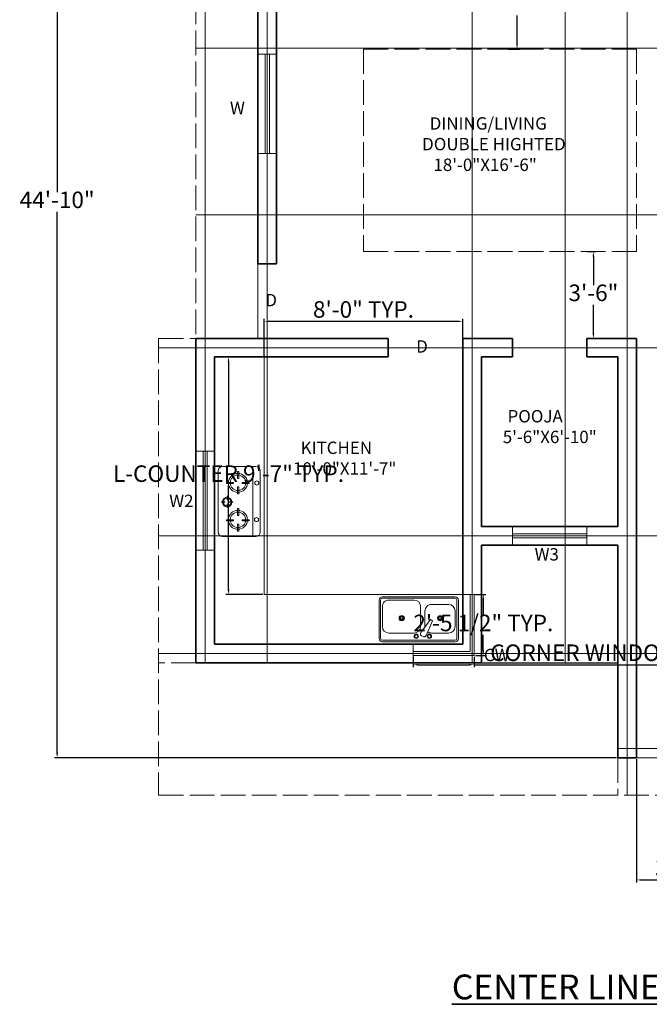
# Model space of a CAD drawing. Units: inches. Extents: x 1070 to 2371, y 645 to 1546.
# Tile 8 of 10: x 1710 to 2015, y 686 to 1162. Entities that reach past the tile are written whole.
import ezdxf

# ---------------------------------------------------------------- set-up
doc = ezdxf.new("R2010")
doc.units = ezdxf.units.IN
doc.linetypes.add('ACAD_ISO02W100', pattern=[15, 12, -3])
for name, color, linetype, lineweight in [('A-ANNO-DIMS', 2, 'Continuous', 18), ('A-ANNO-TEXT', 7, 'Continuous', 18), ('A-ANNO-TITL', 7, 'Continuous', 35), ('A-AREA-IDEN', 7, 'Continuous', 18), ('A-DOOR', 4, 'Continuous', 18), ('A-EQPM', 9, 'Continuous', 18), ('A-FLOR', 7, 'Continuous', 25), ('A-FLOR-CASE', 9, 'Continuous', 18), ('A-FLOR-FIXT', 9, 'Continuous', 18), ('A-FLOR-OVHD', 8, 'ACAD_ISO02W100', 13), ('A-GLAZ', 4, 'Continuous', 18), ('A-GRID', 8, 'Continuous', 13), ('A-ROOF-OVHD', 8, 'ACAD_ISO02W100', 13), ('A-WALL', 7, 'Continuous', 35)]:
    doc.layers.add(name, color=color, linetype=linetype, lineweight=lineweight)
doc.styles.get("Standard").update_dxf_attribs({"font": 'arial.ttf'})
doc.dimstyles.new('ISO-25', dxfattribs={"dimtxt": 8, "dimasz": 2.5, "dimexe": 1.25, "dimexo": 0.625, "dimtad": 1, "dimtih": 1, "dimtoh": 1, "dimdec": 1, "dimlunit": 3, "dimtxsty": 'Standard', "dimcen": 2.5, "dimadec": 0, "dimazin": 0, "dimtfac": 1, "dimtdec": 1, "dimtmove": 0, "dimatfit": 3, "dimfxl": 1, "dimarcsym": 0})

# ---------------------------------------------------------------- blocks, each defined once
blk = doc.blocks.new('A$C51B36FC3')
at = {"linetype": 'ByBlock'}
for p, q in [((0, 421.4), (0, 33)), ((15, 421.4), (15, 33)), ((767.9, 454.4), (33, 454.4)), ((767.9, 439.4), (33, 439.4)), ((357.3, 402.3), (372.7, 393.4)), ((785.9, 33), (785.9, 421.4)), ((800.9, 33), (800.9, 421.4)), ((33, 143.2), (33, 300.3)), ((99.1, 366.3), (271.4, 366.3)), ((325.7, 391), (261.9, 241.3)), ((281, 230.3), (378.7, 360.4)), ((337.5, 299.4), (337.5, 143.2)), ((381.5, 99.1), (381.5, 300.3)), ((447.6, 366.3), (701.8, 366.3)), ((767.9, 300.3), (767.9, 99.1)), ((167.7, 217.2), (157.7, 218.2)), ((167.7, 213.8), (157.8, 212.7)), ((168.5, 220.9), (159, 224.1)), ((168.6, 210), (159.2, 206.6)), ((169.7, 223.8), (161, 228.6)), ((170.1, 206.9), (161.5, 201.7)), ((171.7, 226.6), (164.2, 233.2)), ((172.4, 203.8), (165.3, 196.8)), ((174.6, 229.3), (168.8, 237.4)), ((175, 201.7), (169.3, 193.4)), ((178.2, 231.2), (174.5, 240.5)), ((179.3, 199.6), (176.3, 190.1)), ((181.4, 232.2), (179.7, 242)), ((185.3, 232.4), (185.8, 242.4)), ((188.6, 199.3), (191.1, 189.6)), ((189.3, 231.7), (192.3, 241.3)), ((192, 200.6), (196.5, 191.7)), ((193.1, 230.1), (198.2, 238.7)), ((195.5, 202.9), (202.1, 195.4)), ((196, 227.8), (203, 235)), ((198.3, 206.1), (206.6, 200.5)), ((199, 224.1), (207.6, 229.1)), ((200.1, 209.6), (209.5, 206)), ((200.4, 221), (209.9, 224.1)), ((201, 212.9), (210.9, 211.3)), ((201.2, 216.9), (211.2, 217.6)), ((261.9, 241.3), (281, 230.3)), ((555.9, 217.2), (546, 218.2)), ((556, 213.8), (546, 212.7)), ((556.7, 220.9), (547.2, 224.1)), ((556.8, 210), (547.4, 206.6)), ((558, 223.8), (549.2, 228.6)), ((558.3, 206.9), (549.8, 201.7)), ((560, 226.6), (552.4, 233.2)), ((560.7, 203.8), (553.6, 196.8)), ((562.9, 229.3), (557.1, 237.4)), ((563.2, 201.7), (557.6, 193.4)), ((566.5, 231.2), (562.8, 240.5)), ((567.6, 199.6), (564.5, 190.1)), ((569.7, 232.2), (567.9, 242)), ((573.5, 232.4), (574, 242.4)), ((576.9, 199.3), (579.4, 189.6)), ((577.6, 231.7), (580.5, 241.3)), ((580.3, 200.6), (584.8, 191.7)), ((581.3, 230.1), (586.4, 238.7)), ((583.7, 202.9), (590.3, 195.4)), ((584.3, 227.8), (591.2, 235)), ((586.6, 206.1), (594.8, 200.5)), ((587.2, 224.1), (595.9, 229.1)), ((588.4, 209.6), (597.7, 206)), ((588.6, 221), (598.1, 224.1)), ((589.3, 212.9), (599.2, 211.3)), ((589.5, 216.9), (599.4, 217.6)), ((184.7, 198.8), (184.8, 188.8)), ((572.9, 198.8), (573.1, 188.8)), ((33, 15), (767.9, 15)), ((33, 0), (767.9, 0)), ((271.4, 77.1), (99.1, 77.1)), ((701.8, 33), (447.6, 33))]:
    blk.add_line(p, q, dxfattribs=at)
for centre, radius in [((293.4, 399.4), 22), ((293.4, 399.4), 16), ((425.6, 399.4), 22), ((425.6, 399.4), 16), ((184.4, 215.6), 26.8), ((184.4, 215.6), 16.8), ((184.4, 215.6), 11.8), ((572.7, 215.6), 26.8), ((572.7, 215.6), 16.8), ((572.7, 215.6), 11.8)]:
    blk.add_circle(centre, radius, dxfattribs=at)
for centre, radius, start, end in [((33, 421.4), 33, 90, 180), ((33, 421.4), 18, 90, 180), ((346.3, 383.2), 22, 60, 159.46232), ((767.9, 421.4), 33, 0, 90), ((767.9, 421.4), 18, 0, 90), ((99.1, 300.3), 66.1, 90, 180), ((271.4, 300.3), 66.1, 56.60703, 90), ((361.7, 374.4), 22, 320.53768, 60), ((447.6, 300.3), 66.1, 90, 180), ((701.8, 300.3), 66.1, 0, 90), ((99.1, 143.2), 66.1, 180, 270), ((271.4, 143.2), 66.1, 270, 0), ((33, 33), 33, 180, 270), ((33, 33), 18, 180, 270), ((447.6, 99.1), 66.1, 180, 270), ((701.8, 99.1), 66.1, 270, 0), ((767.9, 33), 33, 270, 0), ((767.9, 33), 18, 270, 0)]:
    blk.add_arc(centre, radius, start, end, dxfattribs=at)
blk = doc.blocks.new('A$C2A3C6842')
for p, q in [((45, 432), (675, 432)), ((0, 45), (0, 387)), ((162, 347), (173, 347)), ((162, 276), (162, 347)), ((173, 347), (173, 276)), ((298, 342), (298, 336)), ((334, 342), (298, 342)), ((298, 336), (334, 336)), ((334, 336), (334, 342)), ((352, 363), (352, 399)), ((352, 399), (357, 399)), ((357, 363), (352, 363)), ((357, 319), (352, 319)), ((352, 319), (352, 283)), ((357, 399), (357, 363)), ((357, 283), (357, 319)), ((379, 336), (379, 342)), ((379, 342), (414, 342)), ((414, 336), (379, 336)), ((414, 342), (414, 336)), ((545, 347), (556, 347)), ((545, 276), (545, 347)), ((556, 347), (556, 276)), ((720, 387), (720, 45)), ((55, 233), (55, 221)), ((127, 233), (55, 233)), ((55, 221), (127, 221)), ((127, 221), (127, 233)), ((173, 276), (162, 276)), ((216, 221), (216, 233)), ((216, 233), (287, 233)), ((287, 221), (216, 221)), ((287, 233), (287, 221)), ((352, 283), (357, 283)), ((438, 233), (438, 221)), ((510, 233), (438, 233)), ((438, 221), (510, 221)), ((510, 221), (510, 233)), ((556, 276), (545, 276)), ((598, 233), (670, 233)), ((598, 221), (598, 233)), ((670, 221), (598, 221)), ((670, 233), (670, 221)), ((173, 187), (162, 187)), ((162, 187), (162, 115)), ((162, 115), (173, 115)), ((173, 115), (173, 187)), ((556, 187), (545, 187)), ((545, 187), (545, 115)), ((545, 115), (556, 115)), ((556, 115), (556, 187)), ((1, 77), (720, 77)), ((675, 0), (45, 0))]:
    blk.add_line(p, q)
at = {"extrusion": (0, -1e-16, -1)}
for centre, major_axis, start_param, end_param in [((45, 387), (31.8, 31.8), 3.926991, 5.497787), ((172, 230), (-97.3, 0.1), -0.001099, 6.282086), ((552, 230), (-97.3, 0.1), -0.001099, 6.282086), ((174, 39), (-14.8, 14.8), 5.497787, 11.780972)]:
    blk.add_ellipse(centre, major_axis=major_axis, ratio=1, start_param=start_param, end_param=end_param, dxfattribs=at)
at = {"extrusion": (0, 1e-16, -1)}
blk.add_ellipse((675, 387), major_axis=(-31.8, 31.8), ratio=1, start_param=0.785398, end_param=2.356194, dxfattribs=at)
at = {"extrusion": (-1e-16, -4e-16, -1)}
for centre in [(172, 230), (552, 230)]:
    blk.add_ellipse(centre, major_axis=(-79.3, 0), ratio=1, start_param=-0.0002116186602152, end_param=6.282973688519371, dxfattribs=at)
at = {"extrusion": (-1e-16, -1e-16, -1)}
blk.add_ellipse((355, 340), major_axis=(48.7, 0.1), ratio=1, start_param=3.144125, end_param=9.42731, dxfattribs=at)
at = {"extrusion": (-1e-16, 0, -1)}
for centre, major_axis, start_param, end_param in [((355, 340), (-39.7, 0), -0.000334, 6.282851), ((45, 45), (-31.8, 31.8), 3.926991, 5.497787)]:
    blk.add_ellipse(centre, major_axis=major_axis, ratio=1, start_param=start_param, end_param=end_param, dxfattribs=at)
at = {"extrusion": (2e-16, -2e-16, -1)}
blk.add_ellipse((551, 36), major_axis=(14.8, 14.8), ratio=1, start_param=3.926991, end_param=10.210176, dxfattribs=at)
at = {"extrusion": (-2e-16, 1e-16, -1)}
blk.add_ellipse((675, 45), major_axis=(31.8, 31.8), ratio=1, start_param=0.785398, end_param=2.356194, dxfattribs=at)
at = {"text_generation_flag": 4, "flags": 9}
for tag in ['XSIZE', 'YSIZE']:
    blk.add_attdef(tag, (361, 265), '', height=0.45, rotation=180, dxfattribs=at)
blk = doc.blocks.new('*D15')
at = {"layer": 'A-ANNO-DIMS', "color": 0, "lineweight": -2, "transparency": 16777216}
for p, q in [((1984.57, 1049.77), (1988.94, 1049.77)), ((1987.69, 1047.27), (1987.69, 1033.48)), ((1987.69, 1010.27), (1987.69, 1024.06)), ((1985.17, 1007.77), (1988.94, 1007.77))]:
    blk.add_line(p, q, dxfattribs=at)
at = {"layer": 'A-ANNO-DIMS', "color": 0, "transparency": 16777216}
for points in [[(1987.28, 1047.27), (1988.11, 1047.27), (1987.69, 1049.77)], [(1987.28, 1010.27), (1988.11, 1010.27), (1987.69, 1007.77)]]:
    blk.add_solid(points, dxfattribs=at)
at = {"layer": 'Defpoints', "color": 0, "transparency": 16777216}
for p in [(1983.94, 1049.77), (1987.69, 1049.77), (1984.54, 1007.77)]:
    blk.add_point(p, dxfattribs=at)
at = {"layer": 'A-ANNO-DIMS', "color": 0, "transparency": 16777216, "insert": (1987.69, 1028.77), "char_height": 8, "attachment_point": 5}
blk.add_mtext('3\'-6"', dxfattribs=at)
blk = doc.blocks.new('*D16')
at = {"layer": 'A-ANNO-DIMS', "color": 0, "lineweight": -2, "transparency": 16777216}
for p, q in [((1946.48, 1189.77), (1952.04, 1189.77)), ((1950.79, 1187.27), (1950.79, 1173.48)), ((1950.79, 1150.27), (1950.79, 1164.06)), ((1946.48, 1147.77), (1952.04, 1147.77))]:
    blk.add_line(p, q, dxfattribs=at)
at = {"layer": 'A-ANNO-DIMS', "color": 0, "transparency": 16777216}
for points in [[(1950.37, 1187.27), (1951.21, 1187.27), (1950.79, 1189.77)], [(1950.37, 1150.27), (1951.21, 1150.27), (1950.79, 1147.77)]]:
    blk.add_solid(points, dxfattribs=at)
at = {"layer": 'Defpoints', "color": 0, "transparency": 16777216}
for p in [(1945.86, 1189.77), (1950.79, 1189.77), (1945.86, 1147.77)]:
    blk.add_point(p, dxfattribs=at)
at = {"layer": 'A-ANNO-DIMS', "color": 0, "transparency": 16777216, "insert": (1950.79, 1168.77), "char_height": 8, "attachment_point": 5}
blk.add_mtext('3\'-6"', dxfattribs=at)
blk = doc.blocks.new('GLAZ-CORNER')
for p, q in [((27.5, 29.5), (27.5, 2)), ((29.5, 29.5), (29.5, 0)), ((0, 2), (27.5, 2)), ((0, 0), (29.5, 0))]:
    blk.add_line(p, q)
blk = doc.blocks.new('GLAZ-36IN')
for p, q in [((0, 2), (36, 2)), ((0, 0), (36, 0))]:
    blk.add_line(p, q)
blk = doc.blocks.new('GLAZ-48IN')
for p, q in [((0, 48), (0, 0)), ((2, 48), (2, 0))]:
    blk.add_line(p, q)
blk = doc.blocks.new('COUNTER-L-KITCHEN')
for p, q in [((0, 115), (0, 0)), ((0, 0), (96, 0))]:
    blk.add_line(p, q)
blk = doc.blocks.new('*D37')
at = {"layer": 'A-ANNO-DIMS', "color": 0, "lineweight": -2, "transparency": 16777216}
for p, q in [((1900.54, 853.65), (1900.54, 848.6)), ((1930.04, 853.65), (1930.04, 848.6)), ((1903.04, 849.85), (1927.54, 849.85)), ((1930.04, 849.85), (2104.79, 849.85))]:
    blk.add_line(p, q, dxfattribs=at)
at = {"layer": 'A-ANNO-DIMS', "color": 0, "transparency": 16777216}
for points in [[(1903.04, 850.26), (1903.04, 849.43), (1900.54, 849.85)], [(1927.54, 850.26), (1927.54, 849.43), (1930.04, 849.85)]]:
    blk.add_solid(points, dxfattribs=at)
at = {"layer": 'Defpoints', "color": 0, "transparency": 16777216}
for p in [(1900.54, 854.27), (1930.04, 854.27), (1930.04, 849.85)]:
    blk.add_point(p, dxfattribs=at)
at = {"layer": 'A-ANNO-DIMS', "color": 0, "transparency": 16777216, "insert": (2018.67, 854.61), "char_height": 8, "attachment_point": 5}
blk.add_mtext('CORNER WINDOW 2\'-5 1/2" TYP.', dxfattribs=at)
blk = doc.blocks.new('*D38')
at = {"layer": 'A-ANNO-DIMS', "color": 0, "lineweight": -2, "transparency": 16777216}
for p, q in [((1930.67, 883.77), (1935.72, 883.77)), ((1934.47, 881.27), (1934.47, 873.78)), ((1934.47, 856.77), (1934.47, 864.26)), ((1930.67, 854.27), (1935.72, 854.27))]:
    blk.add_line(p, q, dxfattribs=at)
at = {"layer": 'A-ANNO-DIMS', "color": 0, "transparency": 16777216}
for points in [[(1934.05, 881.27), (1934.89, 881.27), (1934.47, 883.77)], [(1934.05, 856.77), (1934.89, 856.77), (1934.47, 854.27)]]:
    blk.add_solid(points, dxfattribs=at)
at = {"layer": 'Defpoints', "color": 0, "transparency": 16777216}
for p in [(1930.04, 883.77), (1934.47, 883.77), (1930.04, 854.27)]:
    blk.add_point(p, dxfattribs=at)
at = {"layer": 'A-ANNO-DIMS', "color": 0, "transparency": 16777216, "insert": (1934.47, 869.02), "char_height": 8, "attachment_point": 5}
blk.add_mtext('2\'-5 1/2" TYP.', dxfattribs=at)
blk = doc.blocks.new('*D45')
at = {"layer": 'A-ANNO-DIMS', "color": 0, "lineweight": -2, "transparency": 16777216}
for p, q in [((1827.92, 998.77), (1810.04, 998.77)), ((1811.29, 996.27), (1811.29, 946.04)), ((1811.29, 886.27), (1811.29, 936.51)), ((1827.92, 883.77), (1810.04, 883.77))]:
    blk.add_line(p, q, dxfattribs=at)
at = {"layer": 'A-ANNO-DIMS', "color": 0, "transparency": 16777216}
for points in [[(1810.88, 996.27), (1811.71, 996.27), (1811.29, 998.77)], [(1810.88, 886.27), (1811.71, 886.27), (1811.29, 883.77)]]:
    blk.add_solid(points, dxfattribs=at)
at = {"layer": 'Defpoints', "color": 0, "transparency": 16777216}
for p in [(1811.29, 998.77), (1828.54, 998.77), (1828.54, 883.77)]:
    blk.add_point(p, dxfattribs=at)
at = {"layer": 'A-ANNO-DIMS', "color": 0, "transparency": 16777216, "insert": (1811.29, 941.27), "char_height": 8, "attachment_point": 5}
blk.add_mtext('L-COUNTER 9\'-7" TYP.', dxfattribs=at)
blk = doc.blocks.new('*D46')
at = {"layer": 'A-ANNO-DIMS', "color": 0, "lineweight": -2, "transparency": 16777216}
for p, q in [((1828.54, 999.4), (1828.54, 1017.27)), ((1831.04, 1016.02), (1922.04, 1016.02)), ((1924.54, 999.4), (1924.54, 1017.27))]:
    blk.add_line(p, q, dxfattribs=at)
at = {"layer": 'A-ANNO-DIMS', "color": 0, "transparency": 16777216}
for points in [[(1831.04, 1016.44), (1831.04, 1015.61), (1828.54, 1016.02)], [(1922.04, 1016.44), (1922.04, 1015.61), (1924.54, 1016.02)]]:
    blk.add_solid(points, dxfattribs=at)
at = {"layer": 'Defpoints', "color": 0, "transparency": 16777216}
for p in [(1924.54, 1016.02), (1828.54, 998.77), (1924.54, 998.77)]:
    blk.add_point(p, dxfattribs=at)
at = {"layer": 'A-ANNO-DIMS', "color": 0, "transparency": 16777216, "insert": (1876.54, 1020.73), "char_height": 8, "attachment_point": 5}
blk.add_mtext('8\'-0" TYP.', dxfattribs=at)
blk = doc.blocks.new('*D51')
at = {"layer": 'A-ANNO-DIMS', "color": 0, "lineweight": -2, "transparency": 16777216}
for p, q in [((2008.54, 804.15), (2008.54, 744.47)), ((2050.54, 804.15), (2050.54, 744.47)), ((2011.04, 745.72), (2048.04, 745.72))]:
    blk.add_line(p, q, dxfattribs=at)
at = {"layer": 'A-ANNO-DIMS', "color": 0, "transparency": 16777216}
for points in [[(2011.04, 746.14), (2011.04, 745.31), (2008.54, 745.72)], [(2048.04, 746.14), (2048.04, 745.31), (2050.54, 745.72)]]:
    blk.add_solid(points, dxfattribs=at)
at = {"layer": 'Defpoints', "color": 0, "transparency": 16777216}
for p in [(2008.54, 804.77), (2050.54, 804.77), (2050.54, 745.72)]:
    blk.add_point(p, dxfattribs=at)
at = {"layer": 'A-ANNO-DIMS', "color": 0, "transparency": 16777216, "insert": (2029.54, 750.43), "char_height": 8, "attachment_point": 5}
blk.add_mtext('3\'-6"', dxfattribs=at)
blk = doc.blocks.new('*D53')
at = {"layer": 'A-ANNO-DIMS', "color": 0, "lineweight": -2, "transparency": 16777216}
for p, q in [((1786.92, 1342.77), (1727.24, 1342.77)), ((1728.49, 1340.27), (1728.49, 1078.48)), ((1728.49, 807.27), (1728.49, 1069.06)), ((1998.92, 804.77), (1727.24, 804.77))]:
    blk.add_line(p, q, dxfattribs=at)
at = {"layer": 'A-ANNO-DIMS', "color": 0, "transparency": 16777216}
for points in [[(1728.08, 1340.27), (1728.91, 1340.27), (1728.49, 1342.77)], [(1728.08, 807.27), (1728.91, 807.27), (1728.49, 804.77)]]:
    blk.add_solid(points, dxfattribs=at)
at = {"layer": 'Defpoints', "color": 0, "transparency": 16777216}
for p in [(1787.54, 1342.77), (1728.49, 804.77), (1999.54, 804.77)]:
    blk.add_point(p, dxfattribs=at)
at = {"layer": 'A-ANNO-DIMS', "color": 0, "transparency": 16777216, "insert": (1728.49, 1073.77), "char_height": 8, "attachment_point": 5}
blk.add_mtext('44\'-10"', dxfattribs=at)

msp = doc.modelspace()

# ---------------------------------------------------------------- linework, layer by layer
at = {"layer": 'A-DOOR'}
for p, q in [((1825.54, 1043.77), (1825.54, 1007.77)), ((2008.54, 804.77), (2050.54, 804.77))]:
    msp.add_line(p, q, dxfattribs=at)
at = {"layer": 'A-FLOR'}
msp.add_line((1933.54, 850.77), (1999.54, 850.77), dxfattribs=at)
at = {"layer": 'A-FLOR-OVHD'}
for p, q in [((1876.54, 1147.77), (2008.54, 1147.77)), ((1876.54, 1147.77), (1876.54, 1049.77)), ((2008.54, 1147.77), (2008.54, 1049.77)), ((1876.54, 1049.77), (2008.54, 1049.77))]:
    msp.add_line(p, q, dxfattribs=at)
at = {"layer": 'A-GLAZ'}
for p, q in [((1834.54, 1145.27), (1825.54, 1145.27)), ((1834.54, 1097.27), (1825.54, 1097.27)), ((1804.54, 953.27), (1795.54, 953.27)), ((1948.54, 916.77), (1948.54, 907.77)), ((1984.54, 916.77), (1984.54, 907.77)), ((1804.54, 905.27), (1795.54, 905.27)), ((1924.54, 883.77), (1933.54, 883.77)), ((1900.54, 859.77), (1900.54, 850.77))]:
    msp.add_line(p, q, dxfattribs=at)
at = {"layer": 'A-GRID'}
for p, q in [((1800.04, 850.77), (1800.04, 1478.99)), ((1830.04, 850.77), (1830.04, 1478.99)), ((1929.04, 850.77), (1929.04, 1478.99)), ((1974.04, 850.77), (1974.04, 1478.99)), ((2004.04, 786.77), (2004.04, 1478.99)), ((1795.54, 1148.27), (2293.02, 1148.27)), ((1795.54, 1067.56), (2293.02, 1067.56)), ((1777.54, 1003.27), (2293.02, 1003.27)), ((1777.54, 912.27), (2293.02, 912.27)), ((1777.54, 855.27), (2293.02, 855.27)), ((1999.54, 809.27), (2293.02, 809.27))]:
    msp.add_line(p, q, dxfattribs=at)
at = {"layer": 'A-ROOF-OVHD'}
for p, q in [((1795.54, 1171.77), (1795.54, 1007.77)), ((1777.54, 1007.77), (1795.54, 1007.77)), ((1777.54, 1007.77), (1777.54, 786.77)), ((1795.54, 850.77), (1777.54, 850.77)), ((1999.54, 804.77), (1999.54, 786.77)), ((1777.54, 786.77), (2189.54, 786.77))]:
    msp.add_line(p, q, dxfattribs=at)
at = {"layer": 'A-WALL'}
for p, q in [((1834.54, 1198.77), (1834.54, 1043.77)), ((1825.54, 1189.77), (1825.54, 1043.77)), ((1825.54, 1043.77), (1834.54, 1043.77)), ((1795.54, 1007.77), (1888.54, 1007.77)), ((1795.54, 1007.77), (1795.54, 850.77)), ((1888.54, 1007.77), (1888.54, 998.77)), ((1924.54, 1007.77), (1948.54, 1007.77)), ((1924.54, 1007.77), (1924.54, 859.77)), ((1948.54, 998.77), (1948.54, 1007.77)), ((1984.54, 1007.77), (2008.54, 1007.77)), ((1984.54, 998.77), (1984.54, 1007.77)), ((2008.54, 1007.77), (2008.54, 804.77)), ((1804.54, 998.77), (1888.54, 998.77)), ((1804.54, 998.77), (1804.54, 859.77)), ((1933.54, 998.77), (1948.54, 998.77)), ((1933.54, 998.77), (1933.54, 916.77)), ((1984.54, 998.77), (1999.54, 998.77)), ((1999.54, 998.77), (1999.54, 916.77)), ((1933.54, 916.77), (1999.54, 916.77)), ((1933.54, 907.77), (1999.54, 907.77)), ((1933.54, 907.77), (1933.54, 850.77)), ((1999.54, 907.77), (1999.54, 804.77)), ((1804.54, 859.77), (1924.54, 859.77)), ((1795.54, 850.77), (1933.54, 850.77)), ((1999.54, 804.77), (2008.54, 804.77))]:
    msp.add_line(p, q, dxfattribs=at)

# ---------------------------------------------------------------- block references
at = {"layer": 'A-EQPM', "xscale": 0.0470524325747904, "yscale": 0.0470524325747904, "zscale": 0.0470524325747904, "rotation": 90}
msp.add_blockref('A$C2A3C6842', (1826.69, 911.88), dxfattribs=at)
at = {"layer": 'A-FLOR-CASE'}
msp.add_blockref('COUNTER-L-KITCHEN', (1828.54, 883.77), dxfattribs=at)
at = {"layer": 'A-FLOR-FIXT', "xscale": 0.0478318492028633, "yscale": 0.0478318492028633, "zscale": 0.0478318492028633, "rotation": 180}
msp.add_blockref('A$C51B36FC3', (1922.42, 882.72), dxfattribs=at)
at = {"layer": 'A-GLAZ', "rotation": 180}
msp.add_blockref('GLAZ-48IN', (1831.05, 1145.27), dxfattribs=at)
at = {"layer": 'A-GLAZ'}
for name, p in [('GLAZ-48IN', (1799.04, 905.27)), ('GLAZ-36IN', (1948.54, 911.27)), ('GLAZ-CORNER', (1900.54, 854.27))]:
    msp.add_blockref(name, p, dxfattribs=at)

# ---------------------------------------------------------------- texts
at = {"layer": 'A-ANNO-TEXT', "char_height": 6, "attachment_point": 1}
for s, insert in [('W', (1812.02, 1122.23)), ('D', (1829.08, 1029.29)), ('D', (1902.02, 1006.87)), ('W2', (1782.66, 932.15)), ('  W3', (1955.61, 906.29)), ('CW', (1934.75, 857.57))]:
    msp.add_mtext_dynamic_manual_height_columns(s, width=20.5094, gutter_width=12.5, heights=[0], dxfattribs=dict(at, insert=insert))
at = {"layer": 'A-ANNO-TITL', "insert": (1919.24, 699.95), "char_height": 12, "attachment_point": 1}
msp.add_mtext_dynamic_manual_height_columns('{\\LCENTER LINE DIAGRAM}', width=357.2187, gutter_width=12.5, heights=[0], dxfattribs=at)
at = {"layer": 'A-AREA-IDEN', "attachment_point": 1}
for s, width, insert, char_height in [('  DINING/LIVING\\PDOUBLE HIGHTED\\P   18\'-0"X16\'-6"', 97.1991, (1904.89, 1114.77), 6), ('   {\\H2.4x;POOJA\\P5\'-6"X6\'-10"}', 37.3938, (1943.9, 973.09), 2.5), ('   KITCHEN\\P 10\'-0"X11\'-7"', 97.1991, (1840.68, 957.82), 6)]:
    msp.add_mtext_dynamic_manual_height_columns(s, width=width, gutter_width=12.5, heights=[0], dxfattribs=dict(at, insert=insert, char_height=char_height))

# ---------------------------------------------------------------- dimensions: what is measured, and where the dimension line sits
at = {"layer": 'A-ANNO-DIMS'}
for base, p1, p2, override, picture, middle in [((1728.49, 804.77), (1787.54, 1342.77), (1999.54, 804.77), {"dimdec": 1, "dimlfac": 1, "dimrnd": 0, "dimzin": 1, "dimdsep": 46, "dimlunit": 4, "dimfrac": 2}, '*D53', (1728.49, 1073.77)), ((1950.79, 1189.77), (1945.86, 1147.77), (1945.86, 1189.77), {"dimclrd": 0, "dimclre": 0, "dimclrt": 0}, '*D16', (1950.79, 1168.77)), ((1987.69, 1049.77), (1984.54, 1007.77), (1983.94, 1049.77), {"dimclrd": 0, "dimclre": 0, "dimclrt": 0}, '*D15', (1987.69, 1028.77))]:
    dim = msp.add_linear_dim(base=base, p1=p1, p2=p2, angle=90, dimstyle='ISO-25', override=override, dxfattribs=at)
    dim.commit()
    dim.dimension.update_dxf_attribs({"geometry": picture, "text_midpoint": middle})
for base, p1, p2, text, picture, middle in [((1924.54, 1016.02), (1828.54, 998.77), (1924.54, 998.77), '<> TYP.', '*D46', (1876.54, 1020.73)), ((1930.04, 849.85), (1900.54, 854.27), (1930.04, 854.27), 'CORNER WINDOW <> TYP.', '*D37', (2018.67, 854.61))]:
    dim = msp.add_linear_dim(base=base, p1=p1, p2=p2, text=text, dimstyle='ISO-25', override={"dimdec": 1, "dimlfac": 1, "dimrnd": 0, "dimzin": 1, "dimdsep": 46, "dimlunit": 4, "dimfrac": 2}, dxfattribs=at)
    dim.commit()
    dim.dimension.update_dxf_attribs({"geometry": picture, "text_midpoint": middle})
for base, p1, p2, text, picture, middle in [((1811.29, 998.77), (1828.54, 883.77), (1828.54, 998.77), 'L-COUNTER <> TYP.', '*D45', (1811.29, 941.27)), ((1934.47, 883.77), (1930.04, 854.27), (1930.04, 883.77), '<> TYP.', '*D38', (1934.47, 869.02))]:
    dim = msp.add_linear_dim(base=base, p1=p1, p2=p2, angle=90, text=text, dimstyle='ISO-25', override={"dimdec": 1, "dimlfac": 1, "dimrnd": 0, "dimzin": 1, "dimdsep": 46, "dimlunit": 4, "dimfrac": 2}, dxfattribs=at)
    dim.commit()
    dim.dimension.update_dxf_attribs({"geometry": picture, "text_midpoint": middle})
dim = msp.add_linear_dim(base=(2050.54, 745.72), p1=(2008.54, 804.77), p2=(2050.54, 804.77), dimstyle='ISO-25', override={"dimdec": 1, "dimlfac": 1, "dimrnd": 0, "dimzin": 1, "dimdsep": 46, "dimlunit": 4, "dimfrac": 2}, dxfattribs=at)
dim.commit()
dim.dimension.update_dxf_attribs({"geometry": '*D51', "text_midpoint": (2029.54, 750.43)})

doc.saveas('drawing.dxf')
